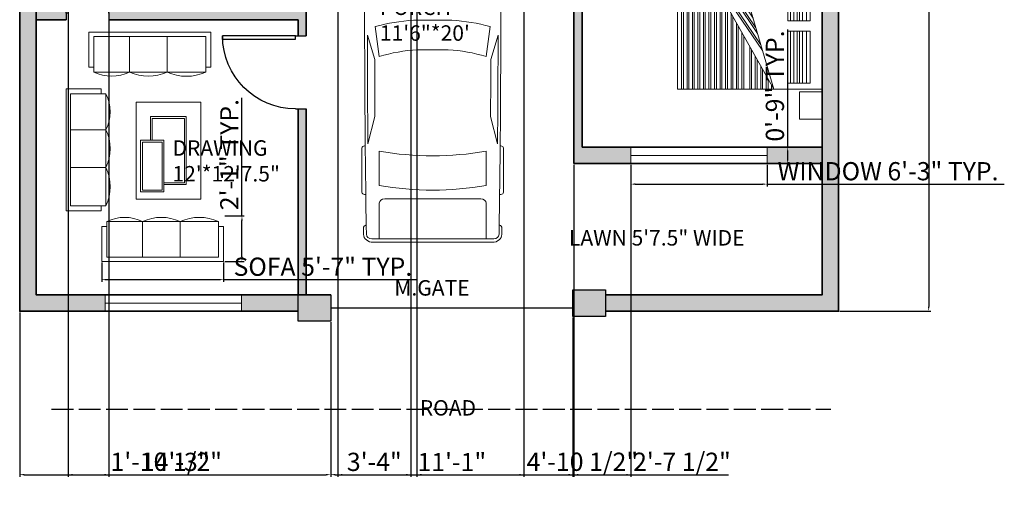
# Model space of a CAD drawing. Units: inches. Extents: x 1698 to 2352, y 1975 to 2732.
# Tile 1 of 4: x 1806 to 2347, y 1975 to 2234. Entities that reach past the tile are written whole.
import ezdxf

# ---------------------------------------------------------------- set-up
doc = ezdxf.new("R2010")
doc.units = ezdxf.units.IN
doc.linetypes.add('ACAD_ISO02W100', pattern=[15, 12, -3])
for name, color, linetype, lineweight in [('A-ANNO-DIMS', 2, 'Continuous', 18), ('A-ANNO-TEXT', 7, 'Continuous', 25), ('A-AREA-IDEN', 7, 'Continuous', 18), ('A-WALL-PATT', 52, 'Continuous', 13), ('C-ROAD', 7, 'ACAD_ISO02W100', 25), ('C-SITE-GATE', 7, 'Continuous', 25), ('car', 171, 'Continuous', 13), ('door', 80, 'Continuous', 25), ('fur', 10, 'Continuous', 18), ('wall', 7, 'Continuous', 35), ('window', 130, 'Continuous', 18)]:
    doc.layers.add(name, color=color, linetype=linetype, lineweight=lineweight)
doc.styles.get("Standard").update_dxf_attribs({"font": 'arial.ttf'})
doc.dimstyles.new('ISO-25', dxfattribs={"dimtxt": 10, "dimasz": 2.5, "dimexe": 1.25, "dimexo": 0.625, "dimtad": 1, "dimdec": 0, "dimlunit": 4, "dimtxsty": 'Standard', "dimcen": 2.5, "dimadec": 0, "dimazin": 0, "dimtfac": 1, "dimtdec": 0, "dimtmove": 0, "dimatfit": 3, "dimfxl": 1, "dimarcsym": 0})

# ---------------------------------------------------------------- blocks, each defined once
blk = doc.blocks.new('*U6')
for p, q in [((46.55, 38.89), (22.35, 38.89)), ((136.7, 38.89), (160.9, 38.89)), ((21.1, 37.41), (21.1, 36.83)), ((47.8, 37.39), (47.8, 37.41)), ((87.99, 31.87), (74.76, 35.92)), ((134.31, 35.6), (119.29, 31.78)), ((135.45, 37.07), (135.45, 37.41)), ((162.15, 37.41), (162.15, 36.77)), ((186.47, -33.5), (186.47, 33.5)), ((188.4, -32.76), (188.4, 32.76)), ((70.03, 31.54), (86.41, 29.35)), ((138.42, 29.35), (157.25, 29.35)), ((186.47, 29.35), (167.01, 29.35)), ((164.52, 26.39), (164.52, -26.39)), ((32.27, 11.63), (36.13, 17.17)), ((36.13, 17.17), (50.94, 17.17)), ((32.12, 9.51), (32.12, 11.15)), ((3.27, 6.13), (0.1, 0.41)), ((29.77, 9.51), (51.68, 9.51)), ((58.92, -10.77), (58.92, 10.77)), ((66.55, -10.53), (66.55, 10.53)), ((82.74, 8.5), (82.74, -8.5)), ((186.47, -10.53), (186.47, 10.53)), ((0, 0), (51.68, 0)), ((0.1, -0.41), (3.27, -6.13)), ((29.77, -9.51), (51.68, -9.51)), ((32.12, -9.51), (32.12, -11.15)), ((32.27, -11.63), (36.13, -17.17)), ((36.13, -17.17), (50.94, -17.17)), ((86.41, -29.35), (70.03, -31.54)), ((87.99, -31.87), (74.76, -35.92)), ((134.31, -35.6), (119.29, -31.78)), ((157.25, -29.35), (138.42, -29.35)), ((167.01, -29.35), (186.47, -29.35)), ((21.1, -37.41), (21.1, -36.83)), ((47.8, -37.39), (47.8, -37.41)), ((135.45, -37.07), (135.45, -37.41)), ((162.15, -37.41), (162.15, -36.77)), ((46.55, -38.89), (22.35, -38.89)), ((136.7, -38.89), (160.9, -38.89))]:
    blk.add_line(p, q)
for centre, major_axis, ratio, start_param, end_param in [((22.35, 37.41), (0, -1.48), 0.842304, 3.141593, 4.712389), ((46.55, 37.41), (0, 1.48), 0.842304, -1.570796, 0), ((136.7, 37.41), (0, -1.48), 0.842304, 3.141593, 4.712389), ((160.9, 37.41), (0, 1.48), 0.842304, -1.570796, 0), ((180.63, 35.84), (0, 2.22), 0.842304, -0.013017, 1.249894), ((64.48, -10556.36), (0, 10595.31), 0.842304, -0.013397, -0.013017), ((183.98, 32.76), (0, -5.25), 0.842304, 1.570796, 3.128196), ((266.03, -27.52), (0, 313.31), 0.842304, 1.367076, 1.39176), ((41.19, -490.86), (0, 528.23), 0.842304, 0.00281, 0.075598), ((64.48, -10555.62), (0, 10593.03), 0.842304, -0.013397, 0.002797), ((64.48, -10555.62), (0, -10591.55), 0.842304, 3.133765, 3.140441), ((183.98, 33.5), (0, -2.96), 0.842304, 1.570796, 3.128196), ((259.18, -27.52), (0, -305.3), 0.842304, 4.528606, 4.561838), ((37.47, -593.96), (0, -623.33), 0.842304, 3.096046, 3.200911), ((134.4, 5.39), (0, -89.78), 0.842304, 4.449482, 4.652344), ((135.29, 5.39), (0, 81.77), 0.842304, 1.245306, 1.50788), ((149.6, 2.8), (0, -79.58), 0.842304, 4.372215, 4.640744), ((95.79, -3666.35), (0, -3698.24), 0.842304, 3.134049, 3.144098), ((17.08, 0), (0, 147.02), 0.842304, 4.511394, 4.913384), ((35.91, 0), (0, 147.02), 0.842304, 4.511394, 4.913384), ((167.01, 26.39), (0, 2.96), 0.842304, 0, 1.570796), ((-204.49, 52.4), (0, -250.96), 0.842304, 1.385369, 1.434372), ((13.04, 17.01), (0, 27.42), 0.842304, 4.435146, 4.718221), ((14.2, 17.01), (0, 27.42), 0.842304, 4.435146, 4.718221), ((50.79, 13.34), (6.34, -0.36), 0.603834, -1.395552, 1.581315), ((32.75, 11.15), (0, 0.74), 0.842304, 0.879714, 1.570796), ((29.77, -46.66), (0, 56.17), 0.842304, 0, 0.590319), ((0.62, 0), (0, -0.74), 0.842304, 4.131459, 5.293319), ((29.77, 46.66), (0, 56.17), 0.842304, 2.551274, 3.141593), ((-204.49, -52.4), (0, 250.96), 0.842304, -1.434372, -1.385369), ((13.04, -17.01), (0, -27.42), 0.842304, 1.564964, 1.848039), ((14.2, -17.01), (0, -27.42), 0.842304, 1.564964, 1.848039), ((134.4, -5.39), (0, -89.78), 0.842304, -1.510751, -1.307889), ((135.29, -5.39), (0, -81.77), 0.842304, -1.50788, -1.245306), ((149.6, -2.8), (0, -79.58), 0.842304, -1.499151, -1.230623), ((32.75, -11.15), (0, -0.74), 0.842304, 4.712389, 5.403472), ((259.18, 27.52), (0, 305.3), 0.842304, 1.721348, 1.754579), ((167.01, -26.39), (0, -2.96), 0.842304, 4.712389, 6.283185), ((266.03, 27.52), (0, 313.31), 0.842304, 1.749832, 1.774517), ((37.47, 593.96), (0, -623.33), 0.842304, -0.059319, 0.045547), ((95.79, 3666.35), (0, -3698.24), 0.842304, -0.002505, 0.007544), ((41.19, 490.86), (0, -528.23), 0.842304, -0.075598, -0.00281), ((22.35, -37.41), (0, 1.48), 0.842304, 1.570796, 3.141593), ((64.48, 10555.62), (0, 10593.03), 0.842304, 3.138796, 3.15499), ((46.55, -37.41), (0, -1.48), 0.842304, 0, 1.570796), ((64.48, 10555.62), (0, -10591.55), 0.842304, 0.001152, 0.007828), ((136.7, -37.41), (0, -1.48), 0.842304, -1.570796, 0), ((160.9, -37.41), (0, 1.48), 0.842304, 3.141593, 4.712389), ((180.63, -35.84), (0, -2.22), 0.842304, -1.249894, 0.013017), ((183.98, -33.5), (0, 2.96), 0.842304, 3.15499, 4.712389), ((183.98, -32.76), (0, -5.25), 0.842304, 0.013397, 1.570796), ((64.48, 10556.36), (0, 10595.31), 0.842304, 3.15461, 3.15499)]:
    blk.add_ellipse(centre, major_axis=major_axis, ratio=ratio, start_param=start_param, end_param=end_param)
at = {"extrusion": (0, 0, -1)}
blk.add_ellipse((50.79, -13.34), major_axis=(6.34, 0.36), ratio=0.603834, start_param=-1.395552, end_param=1.581315, dxfattribs=at)
blk = doc.blocks.new('*U2')
for p, q in [((0, 0), (0, -6)), ((40, 0), (40, -6))]:
    blk.add_line(p, q)
blk.add_lwpolyline([(0, 0), (0, 40), (1.75, 40), (1.75, 0)], close=True)
blk.add_arc((0, 0), 40, 0, 90)
blk = doc.blocks.new('*D8')
at = {"layer": 'A-ANNO-DIMS', "color": 0, "lineweight": -2, "transparency": 16777216}
for p, q in [((2256.62, 2614.26), (2306.74, 2614.26)), ((2305.49, 2611.76), (2305.49, 2076.76)), ((2256.62, 2074.26), (2306.74, 2074.26))]:
    blk.add_line(p, q, dxfattribs=at)
at = {"layer": 'A-ANNO-DIMS', "color": 0, "lineweight": 100, "transparency": 16777216}
for points in [[(2305.07, 2611.76), (2305.9, 2611.76), (2305.49, 2614.26)], [(2305.07, 2076.76), (2305.9, 2076.76), (2305.49, 2074.26)]]:
    blk.add_solid(points, dxfattribs=at)
at = {"layer": 'Defpoints', "color": 0, "lineweight": 100, "transparency": 16777216}
for p in [(2255.99, 2614.26), (2255.99, 2074.26), (2305.49, 2074.26)]:
    blk.add_point(p, dxfattribs=at)
at = {"layer": 'A-ANNO-DIMS', "color": 0, "transparency": 16777216, "insert": (2299.78, 2344.26), "char_height": 10, "attachment_point": 5, "rotation": 90}
blk.add_mtext("45'", dxfattribs=at)
blk = doc.blocks.new('BED-DOUBLE-WITH-NIGHTSTANDS')
for p, q in [((20.55, 70.98), (49.18, 70.98)), ((54.81, 70.98), (83.45, 70.98)), ((20.55, 67.05), (49.18, 67.05)), ((20.55, 65.74), (49.18, 65.74)), ((20.61, 68.69), (49.25, 68.69)), ((54.81, 67.05), (83.45, 67.05)), ((54.81, 65.74), (83.45, 65.74)), ((54.87, 68.69), (83.51, 68.69)), ((20.55, 63.98), (49.18, 63.98)), ((20.55, 62.15), (49.18, 62.15)), ((54.81, 63.98), (83.45, 63.98)), ((54.81, 62.15), (83.45, 62.15)), ((17.28, 32.76), (86.63, 52.89)), ((86.63, 52.89), (27, 19.28)), ((79.34, 48.78), (86.63, 48.78)), ((81.11, 49.78), (86.63, 49.78)), ((84.66, 51.78), (86.63, 51.78)), ((86.25, 52.78), (86.63, 52.78)), ((38.98, 32.41), (56.13, 44.04)), ((40.19, 30.78), (62.43, 45.87)), ((40.75, 29.96), (65.55, 46.77)), ((70.47, 43.78), (86.63, 43.78)), ((74.02, 45.78), (86.63, 45.78)), ((75.79, 46.78), (86.63, 46.78)), ((20.62, 28.13), (35.05, 37.91)), ((35.61, 37.09), (38.16, 38.82)), ((36.83, 35.44), (44.53, 40.67)), ((37.39, 34.62), (47.65, 41.57)), ((38.42, 33.24), (53.01, 43.13)), ((63.38, 39.78), (86.63, 39.78)), ((65.15, 40.78), (86.63, 40.78)), ((68.7, 42.78), (86.63, 42.78)), ((27, 19.28), (17.28, 32.76)), ((21.18, 27.3), (35.61, 37.09)), ((22.4, 25.66), (36.83, 35.44)), ((22.96, 24.83), (37.39, 34.62)), ((23.99, 23.45), (38.42, 33.24)), ((52.14, 33.45), (86.63, 33.45)), ((55.69, 35.45), (86.63, 35.45)), ((57.46, 36.45), (86.63, 36.45)), ((17.28, 32.45), (17.5, 32.45)), ((17.28, 30.45), (18.94, 30.45)), ((17.28, 29.45), (19.66, 29.45)), ((17.28, 27.45), (21.11, 27.45)), ((24.55, 22.62), (38.98, 32.41)), ((25.76, 21), (40.19, 30.78)), ((26.32, 20.17), (40.75, 29.96)), ((41.5, 27.45), (86.63, 27.45)), ((45.05, 29.45), (86.63, 29.45)), ((46.82, 30.45), (86.63, 30.45)), ((50.37, 32.45), (86.63, 32.45)), ((17.28, 26.45), (21.83, 26.45)), ((17.28, 24.45), (23.27, 24.45)), ((17.28, 23.45), (23.99, 23.45)), ((34.41, 23.45), (86.63, 23.45)), ((36.18, 24.45), (86.63, 24.45)), ((39.73, 26.45), (86.63, 26.45)), ((17.28, 21.45), (25.43, 21.45)), ((17.28, 20.45), (26.16, 20.45)), ((17.28, 18.28), (86.63, 18.28)), ((17.28, 17.28), (86.63, 17.28)), ((29.09, 20.45), (86.63, 20.45)), ((30.86, 21.45), (86.63, 21.45)), ((17.28, 15.28), (86.63, 15.28)), ((17.28, 14.28), (86.63, 14.28)), ((17.28, 12.28), (86.63, 12.28)), ((17.28, 11.28), (86.63, 11.28)), ((17.28, 9.28), (86.63, 9.28)), ((17.28, 8.28), (86.63, 8.28)), ((17.28, 6.28), (86.63, 6.28)), ((17.28, 5.28), (86.63, 5.28)), ((17.28, 3.28), (86.63, 3.28)), ((17.28, 2.28), (86.63, 2.28))]:
    blk.add_line(p, q)
for points in [[(0, 79.57), (15.07, 79.57), (15.07, 67), (0, 67)], [(17.28, 79.57), (86.63, 79.57), (86.63, 0), (17.28, 0)], [(88.18, 79.57), (103.25, 79.57), (103.25, 67), (88.18, 67)], [(20.55, 73), (49.18, 73), (49.18, 60.76), (20.55, 60.76)], [(54.81, 73), (83.45, 73), (83.45, 60.76), (54.81, 60.76)]]:
    blk.add_lwpolyline(points, close=True)
blk = doc.blocks.new('SOFA-3-SEAT')
for p, q in [((22.41, 21.86), (22.41, 2.33)), ((43.05, 21.86), (43.05, 2.33)), ((2.74, 19.18), (0, 19.18)), ((0, 19.18), (0, 0)), ((64.21, 19.18), (66.99, 19.18)), ((66.99, 19.18), (66.99, 0)), ((0, 0), (66.99, 0))]:
    blk.add_line(p, q)
blk.add_lwpolyline([(2.74, 2.33), (64.21, 2.33), (64.21, 21.86), (2.74, 21.86)], close=True)
for centre, radius, start, end in [((12.58, 1.63), 22.5, 64.0787, 115.9213), ((32.73, -0.49), 24.61, 65.2107, 114.7893), ((53.63, -1.6), 25.74, 65.7334, 114.2666)]:
    blk.add_arc(centre, radius, start, end)
blk = doc.blocks.new('WIN-75')
blk.add_line((0, 4.5), (75, 4.5))
blk.add_lwpolyline([(0, 9), (75, 9), (75, 0), (0, 0)], close=True)
blk = doc.blocks.new('*D21')
at = {"layer": 'A-ANNO-DIMS', "color": 0, "lineweight": -2, "transparency": 16777216}
for p, q in [((1851.08, 2101), (1851.08, 2090.33)), ((1918.06, 2101), (1918.06, 2090.33)), ((1853.58, 2091.58), (1915.56, 2091.58)), ((1918.06, 2091.58), (2024.64, 2091.58))]:
    blk.add_line(p, q, dxfattribs=at)
at = {"layer": 'A-ANNO-DIMS', "color": 0, "lineweight": 100, "transparency": 16777216}
for points in [[(1853.58, 2092), (1853.58, 2091.16), (1851.08, 2091.58)], [(1915.56, 2092), (1915.56, 2091.16), (1918.06, 2091.58)]]:
    blk.add_solid(points, dxfattribs=at)
at = {"layer": 'Defpoints', "color": 0, "lineweight": 100, "transparency": 16777216}
for p in [(1851.08, 2101.63), (1918.06, 2101.63), (1918.06, 2091.58)]:
    blk.add_point(p, dxfattribs=at)
at = {"layer": 'A-ANNO-DIMS', "color": 0, "transparency": 16777216, "insert": (1972.6, 2097.38), "char_height": 10, "attachment_point": 5}
blk.add_mtext('SOFA 5\'-7" TYP.', dxfattribs=at)
blk = doc.blocks.new('*D22')
at = {"layer": 'A-ANNO-DIMS', "color": 0, "lineweight": -2, "transparency": 16777216}
for p, q in [((1928.11, 2126.52), (1928.11, 2191.39)), ((1918.69, 2126.52), (1929.36, 2126.52)), ((1928.11, 2104.13), (1928.11, 2124.02)), ((1918.69, 2101.63), (1929.36, 2101.63))]:
    blk.add_line(p, q, dxfattribs=at)
at = {"layer": 'A-ANNO-DIMS', "color": 0, "lineweight": 100, "transparency": 16777216}
for points in [[(1927.69, 2124.02), (1928.53, 2124.02), (1928.11, 2126.52)], [(1927.69, 2104.13), (1928.53, 2104.13), (1928.11, 2101.63)]]:
    blk.add_solid(points, dxfattribs=at)
at = {"layer": 'Defpoints', "color": 0, "lineweight": 100, "transparency": 16777216}
for p in [(1918.06, 2126.52), (1928.11, 2126.52), (1918.06, 2101.63)]:
    blk.add_point(p, dxfattribs=at)
at = {"layer": 'A-ANNO-DIMS', "color": 0, "transparency": 16777216, "insert": (1922.46, 2160.21), "char_height": 10, "attachment_point": 5, "rotation": 90}
blk.add_mtext('2\'-1" TYP.', dxfattribs=at)
blk = doc.blocks.new('*D25')
at = {"layer": 'A-ANNO-DIMS', "color": 0, "lineweight": -2, "transparency": 16777216}
for p, q in [((2141.76, 2154.64), (2141.76, 2142.76)), ((2216.76, 2154.64), (2216.76, 2142.76)), ((2144.26, 2144.01), (2214.26, 2144.01)), ((2216.76, 2144.01), (2347.05, 2144.01))]:
    blk.add_line(p, q, dxfattribs=at)
at = {"layer": 'A-ANNO-DIMS', "color": 0, "lineweight": 100, "transparency": 16777216}
for points in [[(2144.26, 2144.43), (2144.26, 2143.6), (2141.76, 2144.01)], [(2214.26, 2144.43), (2214.26, 2143.6), (2216.76, 2144.01)]]:
    blk.add_solid(points, dxfattribs=at)
at = {"layer": 'Defpoints', "color": 0, "lineweight": 100, "transparency": 16777216}
for p in [(2141.76, 2155.26), (2216.76, 2155.26), (2216.76, 2144.01)]:
    blk.add_point(p, dxfattribs=at)
at = {"layer": 'A-ANNO-DIMS', "color": 0, "transparency": 16777216, "insert": (2283.15, 2149.81), "char_height": 10, "attachment_point": 5}
blk.add_mtext('WINDOW 6\'-3" TYP.', dxfattribs=at)
blk = doc.blocks.new('*D26')
at = {"layer": 'A-ANNO-DIMS', "color": 0, "lineweight": -2, "transparency": 16777216}
for p, q in [((2228.01, 2164.26), (2228.01, 2228.97)), ((2217.38, 2164.26), (2229.26, 2164.26)), ((2228.01, 2157.76), (2228.01, 2161.76)), ((2217.38, 2155.26), (2229.26, 2155.26))]:
    blk.add_line(p, q, dxfattribs=at)
at = {"layer": 'A-ANNO-DIMS', "color": 0, "lineweight": 100, "transparency": 16777216}
for points in [[(2227.59, 2161.76), (2228.42, 2161.76), (2228.01, 2164.26)], [(2227.59, 2157.76), (2228.42, 2157.76), (2228.01, 2155.26)]]:
    blk.add_solid(points, dxfattribs=at)
at = {"layer": 'Defpoints', "color": 0, "lineweight": 100, "transparency": 16777216}
for p in [(2216.76, 2164.26), (2228.01, 2164.26), (2216.76, 2155.26)]:
    blk.add_point(p, dxfattribs=at)
at = {"layer": 'A-ANNO-DIMS', "color": 0, "transparency": 16777216, "insert": (2222.27, 2197.86), "char_height": 10, "attachment_point": 5, "rotation": 90}
blk.add_mtext('0\'-9" TYP.', dxfattribs=at)
blk = doc.blocks.new('*D33')
at = {"layer": 'A-ANNO-DIMS', "color": 0, "lineweight": -2, "transparency": 16777216}
for p, q in [((1976.89, 2068.18), (1976.89, 1983.28)), ((2110.02, 2070.81), (2110.02, 1983.28)), ((1979.39, 1984.53), (2107.52, 1984.53))]:
    blk.add_line(p, q, dxfattribs=at)
at = {"layer": 'A-ANNO-DIMS', "color": 0, "lineweight": 100, "transparency": 16777216}
for points in [[(1979.39, 1984.94), (1979.39, 1984.11), (1976.89, 1984.53)], [(2107.52, 1984.94), (2107.52, 1984.11), (2110.02, 1984.53)]]:
    blk.add_solid(points, dxfattribs=at)
at = {"layer": 'Defpoints', "color": 0, "lineweight": 100, "transparency": 16777216}
for p in [(1976.89, 2068.8), (2110.02, 2071.44), (2110.02, 1984.53)]:
    blk.add_point(p, dxfattribs=at)
at = {"layer": 'A-ANNO-DIMS', "color": 0, "transparency": 16777216, "insert": (2043.46, 1990.17), "char_height": 10, "attachment_point": 5}
blk.add_mtext('11\'-1"', dxfattribs=at)
blk = doc.blocks.new('*D34')
at = {"layer": 'A-ANNO-DIMS', "color": 0, "lineweight": -2, "transparency": 16777216}
for p, q in [((1805.99, 2073.64), (1805.99, 1983.28)), ((1976.89, 2068.18), (1976.89, 1983.28)), ((1808.49, 1984.53), (1974.39, 1984.53))]:
    blk.add_line(p, q, dxfattribs=at)
at = {"layer": 'A-ANNO-DIMS', "color": 0, "lineweight": 100, "transparency": 16777216}
for points in [[(1808.49, 1984.94), (1808.49, 1984.11), (1805.99, 1984.53)], [(1974.39, 1984.94), (1974.39, 1984.11), (1976.89, 1984.53)]]:
    blk.add_solid(points, dxfattribs=at)
at = {"layer": 'Defpoints', "color": 0, "lineweight": 100, "transparency": 16777216}
for p in [(1805.99, 2074.26), (1976.89, 2068.8), (1976.89, 1984.53)]:
    blk.add_point(p, dxfattribs=at)
at = {"layer": 'A-ANNO-DIMS', "color": 0, "transparency": 16777216, "insert": (1891.44, 1990.26), "char_height": 10, "attachment_point": 5}
blk.add_mtext('14\'-3"', dxfattribs=at)
blk = doc.blocks.new('*D35')
at = {"layer": 'A-ANNO-DIMS', "color": 0, "lineweight": -2, "transparency": 16777216}
for p, q in [((1832.59, 2238.14), (1832.59, 1983.28)), ((1855.03, 2238.14), (1855.03, 1983.28)), ((1835.09, 1984.53), (1852.53, 1984.53)), ((1855.03, 1984.53), (1915.49, 1984.53))]:
    blk.add_line(p, q, dxfattribs=at)
at = {"layer": 'A-ANNO-DIMS', "color": 0, "lineweight": 100, "transparency": 16777216}
for points in [[(1835.09, 1984.94), (1835.09, 1984.11), (1832.59, 1984.53)], [(1852.53, 1984.94), (1852.53, 1984.11), (1855.03, 1984.53)]]:
    blk.add_solid(points, dxfattribs=at)
at = {"layer": 'Defpoints', "color": 0, "lineweight": 100, "transparency": 16777216}
for p in [(1832.59, 2238.76), (1855.03, 2238.76), (1855.03, 1984.53)]:
    blk.add_point(p, dxfattribs=at)
at = {"layer": 'A-ANNO-DIMS', "color": 0, "transparency": 16777216, "insert": (1886.51, 1990.32), "char_height": 10, "attachment_point": 5}
blk.add_mtext('1\'-10 1/2"', dxfattribs=at)
blk = doc.blocks.new('*D37')
at = {"layer": 'A-ANNO-DIMS', "color": 0, "lineweight": -2, "transparency": 16777216}
for p, q in [((2024.3, 2331.64), (2024.3, 1983.28)), ((2083.04, 2331.64), (2083.04, 1983.28)), ((2026.8, 1984.53), (2080.54, 1984.53)), ((2083.04, 1984.53), (2144.84, 1984.53))]:
    blk.add_line(p, q, dxfattribs=at)
at = {"layer": 'A-ANNO-DIMS', "color": 0, "lineweight": 100, "transparency": 16777216}
for points in [[(2026.8, 1984.94), (2026.8, 1984.11), (2024.3, 1984.53)], [(2080.54, 1984.94), (2080.54, 1984.11), (2083.04, 1984.53)]]:
    blk.add_solid(points, dxfattribs=at)
at = {"layer": 'Defpoints', "color": 0, "lineweight": 100, "transparency": 16777216}
for p in [(2024.3, 2332.26), (2083.04, 2332.26), (2083.04, 1984.53)]:
    blk.add_point(p, dxfattribs=at)
at = {"layer": 'A-ANNO-DIMS', "color": 0, "transparency": 16777216, "insert": (2115.19, 1990.32), "char_height": 10, "attachment_point": 5}
blk.add_mtext('4\'-10 1/2"', dxfattribs=at)
blk = doc.blocks.new('*D39')
at = {"layer": 'A-ANNO-DIMS', "color": 0, "lineweight": -2, "transparency": 16777216}
for p, q in [((1980.85, 2472.64), (1980.85, 1983.28)), ((2020.85, 2472.64), (2020.85, 1983.28)), ((1983.35, 1984.53), (2018.35, 1984.53))]:
    blk.add_line(p, q, dxfattribs=at)
at = {"layer": 'A-ANNO-DIMS', "color": 0, "lineweight": 100, "transparency": 16777216}
for points in [[(1983.35, 1984.94), (1983.35, 1984.11), (1980.85, 1984.53)], [(2018.35, 1984.94), (2018.35, 1984.11), (2020.85, 1984.53)]]:
    blk.add_solid(points, dxfattribs=at)
at = {"layer": 'Defpoints', "color": 0, "lineweight": 100, "transparency": 16777216}
for p in [(1980.85, 2473.26), (2020.85, 2473.26), (2020.85, 1984.53)]:
    blk.add_point(p, dxfattribs=at)
at = {"layer": 'A-ANNO-DIMS', "color": 0, "transparency": 16777216, "insert": (2000.85, 1990.26), "char_height": 10, "attachment_point": 5}
blk.add_mtext('3\'-4"', dxfattribs=at)
blk = doc.blocks.new('*D41')
at = {"layer": 'A-ANNO-DIMS', "color": 0, "lineweight": -2, "transparency": 16777216}
for p, q in [((2110.49, 2154.64), (2110.49, 1983.28)), ((2141.76, 2154.64), (2141.76, 1983.28)), ((2112.99, 1984.53), (2139.26, 1984.53)), ((2141.76, 1984.53), (2195.56, 1984.53))]:
    blk.add_line(p, q, dxfattribs=at)
at = {"layer": 'A-ANNO-DIMS', "color": 0, "lineweight": 100, "transparency": 16777216}
for points in [[(2112.99, 1984.94), (2112.99, 1984.11), (2110.49, 1984.53)], [(2139.26, 1984.94), (2139.26, 1984.11), (2141.76, 1984.53)]]:
    blk.add_solid(points, dxfattribs=at)
at = {"layer": 'Defpoints', "color": 0, "lineweight": 100, "transparency": 16777216}
for p in [(2110.49, 2155.26), (2141.76, 2155.26), (2141.76, 1984.53)]:
    blk.add_point(p, dxfattribs=at)
at = {"layer": 'A-ANNO-DIMS', "color": 0, "transparency": 16777216, "insert": (2169.91, 1990.32), "char_height": 10, "attachment_point": 5}
blk.add_mtext('2\'-7 1/2"', dxfattribs=at)

msp = doc.modelspace()

# ---------------------------------------------------------------- hatches: boundary and pattern name
at = {"layer": 'A-WALL-PATT'}
h = msp.add_hatch(color=256, dxfattribs=at)
h.dxf.hatch_style = 1
h.paths.add_polyline_path([(1910.52, 2614.26), (1805.99, 2614.26), (1805.99, 2549.47), (1814.99, 2549.47), (1814.99, 2605.26), (1910.52, 2605.26)])
h.paths.add_polyline_path([(2084.19, 2614.26), (1972.89, 2614.26), (1972.89, 2605.26), (2026.49, 2605.26), (2084.19, 2605.26)])
h.paths.add_polyline_path([(2255.99, 2614.26), (2146.56, 2614.26), (2146.56, 2605.26), (2148.21, 2605.26), (2186.99, 2605.26), (2246.99, 2605.26), (2246.99, 2546.53), (2255.99, 2546.53)])
h.paths.add_polyline_path([(2191.49, 2605.26), (2186.99, 2605.26), (2186.99, 2595.02), (2191.49, 2595.02)], flags=17)
h.paths.add_polyline_path([(2191.49, 2563.28), (2186.99, 2563.28), (2186.99, 2510.76), (2191.49, 2510.76)])
h.paths.add_polyline_path([(2246.99, 2515.26), (2191.49, 2515.26), (2191.49, 2510.76), (2246.99, 2510.76)])
h.paths.add_polyline_path([(2030.99, 2605.26), (2026.49, 2605.26), (2026.49, 2473.26), (2020.85, 2473.26), (2020.85, 2468.76), (2030.99, 2468.76)])
h.paths.add_polyline_path([(1980.85, 2473.26), (1870.49, 2473.26), (1865.99, 2473.26), (1865.99, 2468.76), (1980.85, 2468.76)])
h.paths.add_polyline_path([(1828.36, 2413.26), (1814.99, 2413.26), (1814.99, 2408.76), (1828.36, 2408.76)])
h.paths.add_polyline_path([(1865.99, 2413.26), (1847.77, 2413.26), (1847.77, 2408.76), (1865.99, 2408.76)])
h.paths.add_polyline_path([(1870.49, 2418.36), (1865.99, 2418.36), (1865.99, 2372.57), (1870.49, 2372.57)])
h.paths.add_polyline_path([(2036.32, 2473.26), (2030.99, 2473.26), (2030.99, 2468.76), (2036.32, 2468.76)])
h.paths.add_polyline_path([(2191.49, 2473.26), (2186.99, 2473.26), (2076.32, 2473.26), (2076.32, 2468.76), (2191.49, 2468.76)])
h.paths.add_polyline_path([(2246.99, 2471.76), (2191.49, 2471.76), (2191.49, 2468.76), (2246.99, 2468.76)])
h.paths.add_polyline_path([(2255.99, 2406.37), (2246.99, 2406.37), (2246.99, 2404.25), (2246.99, 2336.76), (2246.99, 2083.26), (2127.92, 2083.26), (2127.92, 2074.26), (2255.99, 2074.26)])
h.paths.add_polyline_path([(2110.49, 2336.76), (2083.04, 2336.76), (2083.04, 2336.67), (2083.04, 2332.26), (2110.49, 2332.26)])
h.paths.add_polyline_path([(2024.3, 2336.76), (2003.04, 2336.76), (2003.04, 2332.26), (2024.3, 2332.26)])
h.paths.add_polyline_path([(2246.99, 2164.26), (2216.76, 2164.26), (2216.76, 2155.26), (2246.99, 2155.26)], flags=17)
h.paths.add_polyline_path([(1958.99, 2083.26), (1927.89, 2083.26), (1927.89, 2074.26), (1958.99, 2074.26)])
h.paths.add_polyline_path([(1963.49, 2185.34), (1958.99, 2185.34), (1958.99, 2083.26), (1963.49, 2083.26)])
h.paths.add_polyline_path([(1963.49, 2238.76), (1855.03, 2238.76, -0.010403), (1855.05, 2237.79), (1855.05, 2234.26), (1958.99, 2234.26), (1958.99, 2225.34), (1963.49, 2225.34)])
h.paths.add_polyline_path([(1831.56, 2237.79), (1831.56, 2238.76), (1814.99, 2238.76), (1814.99, 2234.26), (1831.56, 2234.26)])
h.paths.add_polyline_path([(1939.87, 2336.76), (1814.99, 2336.76), (1814.99, 2332.26), (1856.99, 2332.26), (1939.87, 2332.26)])
h.paths.add_polyline_path([(1814.99, 2377.93), (1805.99, 2377.93), (1805.99, 2325.81), (1814.99, 2325.81)])
h.paths.add_polyline_path([(1829.84, 2521.26), (1814.99, 2521.26), (1814.99, 2516.76), (1829.84, 2516.76)])
h.paths.add_polyline_path([(2255.99, 2471.76), (2246.99, 2471.76), (2246.99, 2438.09), (2255.99, 2438.09)])
h = msp.add_hatch(color=256, dxfattribs=at)
h.dxf.hatch_style = 1
h.paths.add_polyline_path([(1870.49, 2565.42), (1865.99, 2565.42), (1865.99, 2521.26), (1849.25, 2521.26), (1849.25, 2516.76), (1870.49, 2516.76)])
h.paths.add_polyline_path([(1870.49, 2605.26), (1865.99, 2605.26), (1865.99, 2598.8), (1870.49, 2598.8)])
h.paths.add_polyline_path([(2246.99, 2336.76), (2147.99, 2336.76), (2147.99, 2360.76), (2147.99, 2418.65), (2143.49, 2418.65), (2143.49, 2332.26), (2246.99, 2332.26)])
h.paths.add_polyline_path([(2143.49, 2336.76), (2110.49, 2336.76), (2110.49, 2325.07), (2114.99, 2325.07), (2114.99, 2332.26), (2143.49, 2332.26)])
h.paths.add_polyline_path([(2114.99, 2285.07), (2110.49, 2285.07), (2110.49, 2155.26), (2141.76, 2155.26), (2141.76, 2164.26), (2114.99, 2164.26)])
h.paths.add_polyline_path([(1814.99, 2298.28), (1805.99, 2298.28), (1805.99, 2074.26), (1852.89, 2074.26), (1852.89, 2083.26), (1814.99, 2083.26)])
h = msp.add_hatch(color=256, dxfattribs=at)
h.dxf.hatch_style = 1
h.paths.add_polyline_path([(1976.89, 2083.26), (1958.99, 2083.26), (1958.99, 2068.8), (1976.89, 2068.8)])
h.paths.add_polyline_path([(2127.92, 2085.9), (2110.02, 2085.9), (2110.02, 2071.44), (2127.92, 2071.44)])

# ---------------------------------------------------------------- linework, layer by layer
at = {"layer": 'C-ROAD'}
msp.add_line((1823.47, 2020.48), (2251.76, 2020.48), dxfattribs=at)
at = {"layer": 'C-SITE-GATE'}
msp.add_line((1976.89, 2076.03), (2110.02, 2076.03), dxfattribs=at)
for points in [[(1958.99, 2083.26), (1976.89, 2083.26), (1976.89, 2068.8), (1958.99, 2068.8)], [(2110.02, 2085.9), (2127.92, 2085.9), (2127.92, 2071.44), (2110.02, 2071.44)]]:
    msp.add_lwpolyline(points, close=True, dxfattribs=at)
at = {"layer": 'fur'}
for points in [[(1869.92, 2189.05), (1905.5, 2189.05), (1905.5, 2135.85), (1869.92, 2135.85)], [(1872.45, 2168.07), (1885.28, 2168.07), (1885.28, 2139.72), (1872.45, 2139.72)], [(1873.45, 2167.07), (1884.28, 2167.07), (1884.28, 2140.72), (1873.45, 2140.72)]]:
    msp.add_lwpolyline(points, close=True, dxfattribs=at)
for points in [[(1877.87, 2168.07), (1877.87, 2181.11), (1897.55, 2181.11), (1897.55, 2143.8), (1885.28, 2143.8)], [(1878.87, 2168.07), (1878.87, 2180.11), (1896.55, 2180.11), (1896.55, 2144.8), (1885.28, 2144.8)]]:
    msp.add_lwpolyline(points, dxfattribs=at)
at = {"layer": 'wall'}
for p, q in [((2246.99, 2332.26), (2246.99, 2164.26)), ((2110.49, 2155.26), (2110.49, 2285.07)), ((2114.99, 2164.26), (2114.99, 2285.07)), ((1963.49, 2225.34), (1963.49, 2238.76)), ((1831.56, 2234.26), (1814.99, 2234.26)), ((1958.99, 2234.26), (1855.05, 2234.26)), ((1958.99, 2225.34), (1958.99, 2234.26)), ((1958.99, 2083.26), (1958.99, 2185.34)), ((1963.49, 2083.26), (1963.49, 2185.34)), ((2246.99, 2164.26), (2114.99, 2164.26)), ((2246.99, 2155.26), (2110.49, 2155.26)), ((1814.99, 2083.26), (1958.99, 2083.26))]:
    msp.add_line(p, q, dxfattribs=at)
for points in [[(2127.92, 2074.26), (2255.99, 2074.26), (2255.99, 2614.26), (1805.99, 2614.26), (1805.99, 2074.26), (1958.99, 2074.26)], [(2127.92, 2083.26), (2246.99, 2083.26), (2246.99, 2605.26), (1814.99, 2605.26), (1814.99, 2516.76)], [(1814.99, 2413.26), (1814.99, 2083.26), (1976.89, 2083.26)]]:
    msp.add_lwpolyline(points, dxfattribs=at)

# ---------------------------------------------------------------- block references
at = {"layer": 'car', "rotation": 270}
msp.add_blockref('*U6', (2032.95, 2300.49), dxfattribs=at)
at = {"layer": 'door', "xscale": 0.5871648489528541, "yscale": 0.5871648489528541, "zscale": 0.5871648489528541}
msp.add_blockref('*U2', (1831.56, 2237.79), dxfattribs=at)
at = {"layer": 'door', "xscale": -1, "rotation": 90}
msp.add_blockref('*U2', (1957.49, 2225.34), dxfattribs=at)
at = {"layer": 'fur'}
for name, p, rotation in [('BED-DOUBLE-WITH-NIGHTSTANDS', (2167.42, 2282.85), 270.0000000000057), ('SOFA-3-SEAT', (1831.53, 2196.28), 269.9999999999999)]:
    msp.add_blockref(name, p, dxfattribs=dict(at, rotation=rotation))
at = {"layer": 'fur', "extrusion": (0, 0, -1), "zscale": -1, "rotation": 180}
msp.add_blockref('SOFA-3-SEAT', (-1843.98, 2227.36), dxfattribs=at)
at = {"layer": 'fur'}
msp.add_blockref('SOFA-3-SEAT', (1851.08, 2101.63), dxfattribs=at)
at = {"layer": 'window'}
for p in [(2141.76, 2155.26), (1852.89, 2074.26)]:
    msp.add_blockref('WIN-75', p, dxfattribs=at)

# ---------------------------------------------------------------- texts
at = {"layer": 'A-ANNO-TEXT', "char_height": 8.476, "attachment_point": 1}
for s, insert in [('M.GATE', (2011.86, 2091.3)), ('ROAD', (2025.86, 2025.45))]:
    msp.add_mtext_dynamic_manual_height_columns(s, width=272.6258, gutter_width=42.38, heights=[0], dxfattribs=dict(at, insert=insert))
at = {"layer": 'A-AREA-IDEN', "attachment_point": 1}
for s, insert, char_height in [('PORCH\\P11\'6"*20\'', (2003.94, 2245.32), 8.476), ('DRAWING\\P12\'*12\'7.5"', (1889.96, 2168.07), 8.4756), ('LAWN 5\'7.5" WIDE', (2107.82, 2118.77), 8.4756)]:
    msp.add_mtext_dynamic_manual_height_columns(s, width=272.6258, gutter_width=42.38, heights=[0], dxfattribs=dict(at, insert=insert, char_height=char_height))

# ---------------------------------------------------------------- dimensions: what is measured, and where the dimension line sits
at = {"layer": 'A-ANNO-DIMS'}
dim = msp.add_linear_dim(base=(2305.49, 2074.26), p1=(2255.99, 2614.26), p2=(2255.99, 2074.26), angle=90, dimstyle='ISO-25', override={"dimclrd": 0, "dimclre": 0, "dimclrt": 0}, dxfattribs=at)
dim.commit()
dim.dimension.update_dxf_attribs({"geometry": '*D8', "text_midpoint": (2299.78, 2344.26)})
for base, p1, p2, picture, middle in [((2020.85, 1984.53), (1980.85, 2473.26), (2020.85, 2473.26), '*D39', (2000.85, 1990.26)), ((2083.04, 1984.53), (2024.3, 2332.26), (2083.04, 2332.26), '*D37', (2115.19, 1990.32)), ((1855.03, 1984.53), (1832.59, 2238.76), (1855.03, 2238.76), '*D35', (1886.51, 1990.32)), ((2141.76, 1984.53), (2110.49, 2155.26), (2141.76, 2155.26), '*D41', (2169.91, 1990.32)), ((1976.89, 1984.53), (1805.99, 2074.26), (1976.89, 2068.8), '*D34', (1891.44, 1990.26)), ((2110.02, 1984.53), (1976.89, 2068.8), (2110.02, 2071.44), '*D33', (2043.46, 1990.17))]:
    dim = msp.add_linear_dim(base=base, p1=p1, p2=p2, dimstyle='ISO-25', override={"dimdec": 1, "dimlfac": 1, "dimrnd": 0, "dimzin": 1, "dimdsep": 46, "dimlunit": 4, "dimfrac": 2}, dxfattribs=at)
    dim.commit()
    dim.dimension.update_dxf_attribs({"geometry": picture, "text_midpoint": middle})
for base, p1, p2, picture, middle in [((2228.01, 2164.26), (2216.76, 2155.26), (2216.76, 2164.26), '*D26', (2222.27, 2197.86)), ((1928.11, 2126.52), (1918.06, 2101.63), (1918.06, 2126.52), '*D22', (1922.46, 2160.21))]:
    dim = msp.add_linear_dim(base=base, p1=p1, p2=p2, angle=90, text='<> TYP.', dimstyle='ISO-25', override={"dimdec": 1, "dimlfac": 1, "dimrnd": 0, "dimzin": 1, "dimdsep": 46, "dimlunit": 4, "dimfrac": 2}, dxfattribs=at)
    dim.commit()
    dim.dimension.update_dxf_attribs({"geometry": picture, "text_midpoint": middle})
for base, p1, p2, text, picture, middle in [((2216.76, 2144.01), (2141.76, 2155.26), (2216.76, 2155.26), 'WINDOW <> TYP.', '*D25', (2283.15, 2149.81)), ((1918.06, 2091.58), (1851.08, 2101.63), (1918.06, 2101.63), 'SOFA <> TYP.', '*D21', (1972.6, 2097.38))]:
    dim = msp.add_linear_dim(base=base, p1=p1, p2=p2, text=text, dimstyle='ISO-25', override={"dimdec": 1, "dimlfac": 1, "dimrnd": 0, "dimzin": 1, "dimdsep": 46, "dimlunit": 4, "dimfrac": 2}, dxfattribs=at)
    dim.commit()
    dim.dimension.update_dxf_attribs({"geometry": picture, "text_midpoint": middle})

doc.saveas('drawing.dxf')
